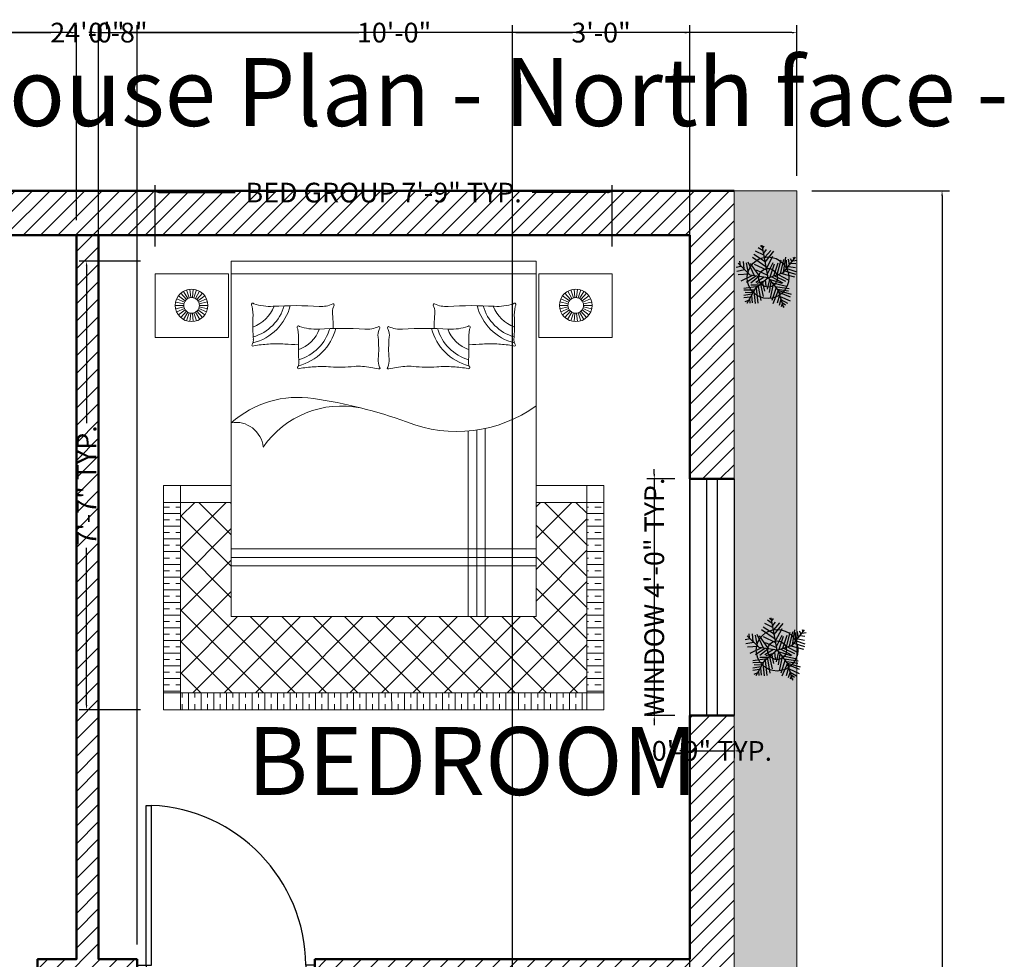
# Model space of a CAD drawing. Units: inches. Extents: x 1265938 to 1266301, y 2357745 to 2358240.
# Tile 4 of 4: x 1266101 to 1266301, y 2358050 to 2358240. Entities that reach past the tile are written whole.
import ezdxf

# ---------------------------------------------------------------- set-up
doc = ezdxf.new("R2010")
doc.units = ezdxf.units.IN
doc.header["$MEASUREMENT"] = 0
for name, color, linetype, lineweight in [('A-ANNO-TEXT', 7, 'Continuous', 25), ('A-AREA-IDEN', 7, 'Continuous', 18), ('A-DOOR', 4, 'Continuous', 25), ('A-FURN', 8, 'Continuous', 18), ('A-WALL-PATT', 8, 'Continuous', 13), ('L-PLNT', 3, 'Continuous', 18), ('L-PLNT-BEDS', 3, 'Continuous', 18), ('L-PLNT-PATT', 3, 'Continuous', 13), ('WALL', 7, 'Continuous', 50), ('WINDOW', 2, 'Continuous', 25), ('YQ_DIM', 3, 'Continuous', 18)]:
    doc.layers.add(name, color=color, linetype=linetype, lineweight=lineweight)
doc.layers.add('Layer2', color=102, linetype='Continuous')
doc.layers.add('RAMP SLOPE', color=8, linetype='Continuous')
doc.styles.get("Standard").update_dxf_attribs({"font": 'arial.ttf'})
doc.styles.add('YQ_DIM', font='SUPEROS.SHX', dxfattribs={"width": 0.8, "bigfont": 'HZDX.SHX'})
doc.dimstyles.new('yqi0', dxfattribs={"dimscale": 0, "dimtxt": 4, "dimasz": 1, "dimexe": 1.5, "dimexo": 3, "dimgap": 0.5, "dimtad": 0, "dimdsep": 46, "dimlunit": 4, "dimtxsty": 'Standard', "dimcen": 0, "dimclrd": 256, "dimclre": 256, "dimclrt": 7, "dimadec": 1, "dimazin": 2, "dimtfac": 1, "dimtix": 1, "dimtmove": 2, "dimatfit": 2, "dimfxl": 1, "dimtolj": 1, "dimtzin": 0, "dimarcsym": 0})

# ---------------------------------------------------------------- blocks, each defined once
blk = doc.blocks.new('WD_WIN4')
for p, q in [((-0.5, 0.5), (0.5, 0.5)), ((-0.5, 0.12), (0.5, 0.12)), ((-0.5, -0.12), (0.5, -0.12)), ((-0.5, -0.5), (0.5, -0.5))]:
    blk.add_line(p, q)
blk = doc.blocks.new('DR_D01')
for p, q in [((-0.45, 0.93), (-0.42, 0.93)), ((-0.45, 0.03), (-0.45, 0.93)), ((-0.42, 0.03), (-0.42, 0.93)), ((-0.5, 0.03), (-0.42, 0.03)), ((-0.5, 0.03), (-0.5, -0.03)), ((-0.45, 0.03), (-0.45, 0)), ((-0.45, 0), (-0.435, 0)), ((-0.435, 0), (-0.435, -0.03)), ((0.435, 0), (0.435, -0.03)), ((0.45, 0), (0.435, 0)), ((0.45, 0.03), (0.45, 0)), ((0.5, 0.03), (0.45, 0.03)), ((0.5, -0.03), (0.5, 0.03)), ((-0.435, -0.03), (-0.5, -0.03)), ((0.435, -0.03), (0.5, -0.03))]:
    blk.add_line(p, q)
blk.add_arc((-0.4602, 0.0206), 0.9103, 0.5915, 87.4664)
blk = doc.blocks.new('Trees - Metric')
at = {"layer": 'Layer2'}
for p, q in [((-221.9198, 1197.3052), (-433.5526, 1338.8594)), ((-258.7244, 1362.456), (-332.3336, 1421.4348)), ((0, 0), (-266.7, 1447.8)), ((-231.1146, 1315.2628), (-166.7002, 1421.4348)), ((-93.091, 489.5342), (-700.3796, 902.3858)), ((-129.8956, 713.6638), (-626.7704, 1032.1544)), ((-185.1152, 1008.5578), (-553.1612, 1185.4942)), ((-194.31, 1102.9442), (-65.4812, 1256.284)), ((-148.3106, 914.1968), (118.5418, 1220.9018)), ((-129.8956, 701.8528), (265.7602, 1185.4942)), ((-74.7014, 418.7444), (219.7608, 961.39)), ((685.8, 228.6), (1219.2, 914.4)), ((689.0258, 230.0224), (790.2448, 914.1968)), ((1121.4862, 925.9824), (1149.0706, 831.6214)), ((-1206.4492, 501.3198), (-1418.082, 465.9376)), ((-800.1, 114.3), (-1333.5, 647.7)), ((-1234.059, 536.7274), (-1252.4486, 737.2604)), ((-1105.2302, 725.4494), (-1077.6458, 395.1732)), ((-976.4268, 666.4706), (-884.4026, 194.6402)), ((-902.8176, 713.6638), (-617.5756, 100.2538)), ((-369.1382, 53.086), (-783.1836, 642.874)), ((-617.5756, 607.4918), (-74.7014, 347.98)), ((-28.6766, 171.0436), (228.9556, 678.2816)), ((100.1268, 41.275), (284.1498, 619.2774)), ((256.5654, 88.4682), (449.7832, 666.4706)), ((412.9786, 147.447), (587.8068, 796.2392)), ((560.197, 182.8292), (698.2206, 819.8358)), ((808.6344, 784.4282), (827.0494, 418.7444)), ((891.4384, 831.6214), (946.658, 572.1096)), ((919.0482, 501.3198), (1222.6798, 454.152)), ((983.4626, 867.0036), (1066.2666, 725.4494)), ((1029.462, 654.685), (1241.0948, 631.0884)), ((1112.2914, 760.8316), (1296.3144, 784.4282)), ((-1031.621, 347.98), (-1399.667, 277.1902)), ((-847.598, 159.2326), (-1326.0578, 135.636)), ((-718.7946, 88.4682), (-1215.644, -147.447)), ((-543.9664, 76.6572), (-967.2066, -206.4512)), ((0, 0), (-800.1, 114.3)), ((-405.9428, 53.086), (-764.794, -241.8334)), ((0, 0), (-571.5, -495.3)), ((-166.7002, 29.4894), (-543.9664, -206.4512)), ((-525.5514, 347.98), (-28.6766, 123.8504)), ((0, 0), (685.8, 228.6)), ((0, 0), (457.2, -571.5)), ((164.5412, 41.275), (661.416, -218.2368)), ((284.1498, 88.4682), (781.0246, -147.447)), ((458.978, 147.447), (891.4384, -88.4682)), ((615.4166, 194.6402), (1185.8752, 41.275)), ((753.4148, 312.5978), (1222.6798, 159.2326)), ((845.439, 418.7444), (1241.0948, 277.1902)), ((-442.7474, -383.3876), (-1086.8406, -477.7486)), ((-387.5278, -324.4088), (-764.794, -324.4088)), ((-166.7002, -147.447), (-507.1618, -253.619)), ((-433.5526, -383.3876), (-323.1134, -1020.3688)), ((-341.5284, -289.0012), (-221.9198, -831.6214)), ((-240.3094, -218.2368), (-157.5054, -595.7062)), ((-120.7008, -88.4682), (-93.091, -371.5766)), ((63.3222, -76.6826), (-37.8714, -513.1308)), ((44.9326, -64.897), (615.4166, -241.8334)), ((127.7366, -159.258), (54.1274, -654.685)), ((228.9556, -289.0012), (90.932, -914.1968)), ((357.759, -430.5554), (164.5412, -1020.3688)), ((192.151, -230.0224), (817.8292, -371.5766)), ((311.7596, -383.3876), (937.4378, -477.7486)), ((-718.7946, -737.2604), (-1086.8406, -796.2392)), ((-617.5756, -548.5384), (-1077.6458, -560.324)), ((-783.1836, -867.029), (-1077.6458, -902.4112)), ((-681.9646, -666.496), (-1022.4262, -654.685)), ((-571.5, -495.3), (-952.5, -1143)), ((-737.1842, -784.4536), (-709.5744, -1114.7298)), ((-635.9652, -607.5172), (-580.771, -1150.1374)), ((-525.5514, -465.963), (-451.9422, -1126.5408)), ((458.978, -572.1096), (210.5406, -1161.923)), ((514.1976, -772.6426), (403.7838, -1138.3264)), ((412.9786, -501.3452), (919.0482, -583.9206)), ((457.2, -571.5), (685.8, -1333.5)), ((468.1982, -572.1096), (1029.462, -737.2604)), ((486.5878, -642.8994), (983.4626, -843.4324)), ((541.8074, -831.6214), (992.6574, -1032.1544)), ((-875.2078, -1008.5832), (-1040.8412, -1079.3476)), ((-829.2084, -937.7934), (-810.7934, -1126.5408)), ((578.612, -961.39), (495.7826, -1232.7128)), ((578.612, -973.1756), (873.0488, -1138.3264)), ((624.6114, -1161.923), (587.8068, -1291.6916)), ((624.6114, -1102.9442), (781.0246, -1209.1162)), ((679.8056, -1268.095), (716.6102, -1291.6916))]:
    blk.add_line(p, q, dxfattribs=at)
blk = doc.blocks.new('A$Cbdbf8f2b')
at = {"layer": 'RAMP SLOPE'}
for radius in [7.17, 3.22]:
    blk.add_circle((13.77, 14.11), radius, dxfattribs=at)
at = {"xscale": 0.0077264756515533, "yscale": 0.0077264756515533, "zscale": 0.0077264756515533}
blk.add_blockref('Trees - Metric', (13.77, 14.11), dxfattribs=at)
blk = doc.blocks.new('BED')
h = blk.add_hatch()
h.set_pattern_fill('TRANS', color=256, scale=12, style=0)
h.set_pattern_definition([(360, (4433.967, -9715.0492), (1e-15, 3), []), (360, (4433.967, -9713.5492), (1e-15, 3), [1.5, -1.5])])
h.paths.add_polyline_path([(48, -103), (52, -103), (52, -58), (48, -58)])
h.paths.add_polyline_path([(-48, -58), (-52, -58), (-52, -103), (-48, -103)])
h = blk.add_hatch()
h.set_pattern_fill('ANSI37', color=256, scale=42, angle=-90, style=0)
h.set_pattern_definition([(315, (7787.1367, 4477.8466), (3.7123106, 3.7123106), []), (45, (7787.1367, 4477.8466), (-3.7123106, 3.7123106), [])])
h.paths.add_polyline_path([(-36, -85), (-36, -58), (-48, -58), (-48, -103), (48, -103), (48, -58), (36, -58), (36, -85)])
h = blk.add_hatch()
h.set_pattern_fill('TRANS', color=256, scale=12, angle=-90, style=0)
h.set_pattern_definition([(270, (4433.967, -9715.0492), (3, -1e-15), []), (270, (4435.467, -9715.0492), (3, -1e-15), [1.5, -1.5])])
h.paths.add_polyline_path([(48, -107), (48, -103), (-48, -103), (-48, -107)])
for p, q in [((-36, -1), (36, -1)), ((-36, -85), (-36, -1)), ((36, -1), (36, -85)), ((-54, -4), (-54, -19)), ((-36.64, -4), (-54, -4)), ((-36.64, -4), (-36.64, -19)), ((-36, -4), (36, -4)), ((36.64, -4), (36.64, -19)), ((36.64, -4), (54, -4)), ((54, -4), (54, -19)), ((-46.88, -10.37), (-48.5, -9.2)), ((-46.62, -10.08), (-47.96, -8.6)), ((-46.31, -9.86), (-47.31, -8.13)), ((-45.96, -9.7), (-46.58, -7.8)), ((-45.58, -9.62), (-45.8, -7.63)), ((-45.2, -9.62), (-45, -7.63)), ((-44.82, -9.7), (-44.21, -7.79)), ((-44.47, -9.85), (-43.48, -8.12)), ((-44.16, -10.08), (-42.83, -8.59)), ((-43.9, -10.36), (-42.29, -9.18)), ((43.9, -10.36), (42.29, -9.18)), ((44.16, -10.08), (42.83, -8.59)), ((44.47, -9.85), (43.48, -8.12)), ((44.82, -9.7), (44.21, -7.79)), ((45.2, -9.62), (45, -7.63)), ((45.58, -9.62), (45.8, -7.63)), ((45.96, -9.7), (46.58, -7.8)), ((46.31, -9.86), (47.31, -8.13)), ((46.62, -10.08), (47.96, -8.6)), ((46.88, -10.37), (48.5, -9.2)), ((-47.23, -11.45), (-49.23, -11.45)), ((-47.19, -11.07), (-49.14, -10.66)), ((-47.07, -10.7), (-48.9, -9.89)), ((-43.71, -10.7), (-41.89, -9.88)), ((-43.59, -11.06), (-41.64, -10.64)), ((-43.55, -11.44), (-41.55, -11.44)), ((43.55, -11.44), (41.55, -11.44)), ((43.59, -11.06), (41.64, -10.64)), ((43.71, -10.7), (41.89, -9.88)), ((47.07, -10.7), (48.9, -9.89)), ((47.19, -11.07), (49.14, -10.66)), ((47.23, -11.45), (49.23, -11.45)), ((-47.19, -11.83), (-49.14, -12.25)), ((-47.07, -12.2), (-48.89, -13.01)), ((-46.87, -12.53), (-48.49, -13.71)), ((-46.62, -12.81), (-47.95, -14.3)), ((-46.3, -13.04), (-47.3, -14.77)), ((-45.95, -13.2), (-46.57, -15.1)), ((-45.58, -13.27), (-45.78, -15.26)), ((-45.19, -13.27), (-44.98, -15.26)), ((-44.82, -13.19), (-44.2, -15.09)), ((-44.47, -13.04), (-43.46, -14.77)), ((-44.16, -12.81), (-42.82, -14.29)), ((-43.9, -12.52), (-42.28, -13.7)), ((-43.71, -12.19), (-41.88, -13)), ((-43.59, -11.83), (-41.63, -12.24)), ((43.59, -11.83), (41.63, -12.24)), ((43.71, -12.19), (41.88, -13)), ((43.9, -12.52), (42.28, -13.7)), ((44.16, -12.81), (42.82, -14.29)), ((44.47, -13.04), (43.46, -14.77)), ((44.82, -13.19), (44.2, -15.09)), ((45.19, -13.27), (44.98, -15.26)), ((45.58, -13.27), (45.78, -15.26)), ((45.95, -13.2), (46.57, -15.1)), ((46.3, -13.04), (47.3, -14.77)), ((46.62, -12.81), (47.95, -14.3)), ((46.87, -12.53), (48.49, -13.71)), ((47.07, -12.2), (48.89, -13.01)), ((47.19, -11.83), (49.14, -12.25)), ((-36.64, -19), (-54, -19)), ((36.64, -19), (54, -19)), ((20, -85), (20, -41.14)), ((22, -85), (22, -40.91)), ((24, -85), (24, -40.55)), ((-52, -54), (-52, -107)), ((-52, -54), (-36, -54)), ((-48, -54), (-48, -107)), ((36, -54), (52, -54)), ((48, -54), (48, -107)), ((52, -54), (52, -107)), ((-52, -58), (-36, -58)), ((36, -58), (52, -58)), ((36, -69), (-36, -69)), ((36, -71), (-36, -71)), ((36, -73), (-36, -73)), ((36, -85), (-36, -85)), ((-52, -103), (52, -103)), ((-52, -107), (52, -107))]:
    blk.add_line(p, q)
for centre, radius in [((-45.39, -11.45), 3.84), ((45.39, -11.45), 3.84), ((-45.39, -11.45), 1.84), ((45.39, -11.45), 1.84)]:
    blk.add_circle(centre, radius)
for centre, radius, start, end in [((-30.92, -11.24), 0.328, 35.8976, 208.6272), ((-42.38, -17.5), 12.73, 27.1629, 28.6272), ((-33.8, -8.61), 12.06, 283.8498, 346.0842), ((-33.8, -8.61), 10.71, 286.0319, 344.1205), ((-26.84, 0.13), 11.82, 251.1782, 273.3982), ((-20.92, -99.64), 88.13, 86.2964, 93.3982), ((-14.79, -4.98), 6.73, 266.2964, 294.303), ((-11.92, -11.33), 0.242, 335.7259, 114.303), ((-5.69, -14.14), 6.59, 155.7259, 159.0146), ((11.92, -11.33), 0.242, 65.697, 204.2741), ((5.69, -14.14), 6.59, 20.9854, 24.2741), ((14.79, -4.98), 6.73, 245.697, 273.7036), ((20.92, -99.64), 88.13, 86.6018, 93.7036), ((33.8, -8.61), 12.06, 193.9158, 256.1502), ((33.8, -8.61), 10.71, 195.8795, 253.9681), ((26.84, 0.13), 11.82, 266.6018, 288.8218), ((30.92, -11.24), 0.328, 331.3728, 144.1024), ((42.38, -17.5), 12.73, 151.3728, 152.8371), ((-44.37, -13.89), 13.5, 357.4804, 9.3956), ((-33.8, -8.61), 8.46, 289.8695, 338.9843), ((-8.24, -13.16), 3.86, 159.0146, 186.273), ((-36.64, -16.28), 24.71, 358.5721, 6.273), ((8.24, -13.16), 3.86, 353.727, 20.9854), ((36.64, -16.28), 24.71, 173.727, 181.4279), ((33.8, -8.61), 8.46, 201.0157, 250.1305), ((44.37, -13.89), 13.5, 170.6044, 182.5196), ((10.15, -16.29), 41.07, 177.4804, 184.5075), ((-10.15, -16.29), 41.07, 355.4925, 2.5196), ((-20.16, -16.62), 0.328, 35.8976, 208.6272), ((-31.62, -22.87), 12.73, 27.1629, 28.6272), ((-33.61, -19.26), 13.5, 357.4804, 9.3956), ((-23.04, -13.99), 8.46, 289.8695, 338.9843), ((-23.04, -13.99), 12.06, 283.8498, 346.0842), ((-23.04, -13.99), 10.71, 286.0319, 344.1205), ((-16.08, -5.24), 11.82, 251.1782, 273.3982), ((-10.15, -105.01), 88.13, 86.2964, 93.3982), ((-4.03, -10.35), 6.73, 266.2964, 294.303), ((2.52, -18.53), 3.86, 159.0146, 186.273), ((-1.16, -16.7), 0.242, 335.7259, 114.303), ((5.07, -19.51), 6.59, 155.7259, 159.0146), ((1.16, -16.7), 0.242, 65.697, 204.2741), ((-5.07, -19.51), 6.59, 20.9854, 24.2741), ((-2.52, -18.53), 3.86, 353.727, 20.9854), ((4.03, -10.35), 6.73, 245.697, 273.7036), ((10.15, -105.01), 88.13, 86.6018, 93.7036), ((23.04, -13.99), 12.06, 193.9158, 256.1502), ((23.04, -13.99), 10.71, 195.8795, 253.9681), ((23.04, -13.99), 8.46, 201.0157, 250.1305), ((16.08, -5.24), 11.82, 266.6018, 288.8218), ((20.16, -16.62), 0.328, 331.3728, 144.1024), ((33.61, -19.26), 13.5, 170.6044, 182.5196), ((31.62, -22.87), 12.73, 151.3728, 152.8371), ((-30.88, -20.82), 0.25, 147.6219, 311.9343), ((-32.72, -19.65), 1.93, 327.6219, 339.2246), ((-32.67, -19.67), 1.88, 339.2246, 4.5075), ((-25.16, -53.53), 33, 93.5164, 99.6766), ((-25.27, -51.86), 31.33, 86.4836, 93.5164), ((-21.12, 15.68), 36.34, 266.4836, 271.5234), ((20.91, -21.66), 41.07, 177.4804, 184.5075), ((-25.88, -21.66), 24.71, 354.3784, 6.273), ((25.88, -21.66), 24.71, 173.727, 185.6216), ((-20.91, -21.66), 41.07, 355.4925, 2.5196), ((21.12, 15.68), 36.34, 268.4766, 273.5164), ((25.27, -51.86), 31.33, 86.4836, 93.5164), ((25.16, -53.53), 33, 80.3234, 86.4836), ((30.88, -20.82), 0.25, 228.0657, 32.3781), ((32.67, -19.67), 1.88, 175.4925, 200.7754), ((32.72, -19.65), 1.93, 200.7754, 212.3781), ((-21.91, -25.04), 1.88, 339.2246, 4.5075), ((2.55, -24.46), 3.86, 174.3784, 204.7617), ((-2.55, -24.46), 3.86, 335.2383, 5.6216), ((21.91, -25.04), 1.88, 175.4925, 200.7754), ((-20.12, -26.19), 0.25, 147.6219, 311.9343), ((-21.96, -25.02), 1.93, 327.6219, 339.2246), ((-14.4, -58.9), 33, 93.5164, 99.6766), ((-14.51, -57.23), 31.33, 86.4836, 93.5164), ((-10.35, 10.3), 36.34, 266.4836, 275.306), ((-5.78, -38.98), 13.15, 77.9645, 95.306), ((2.5, -0.17), 26.53, 257.9645, 261.9243), ((-1.09, -26.25), 0.228, 231.9005, 52.8902), ((1.09, -26.25), 0.228, 127.1098, 308.0995), ((-2.5, -0.17), 26.53, 278.0757, 282.0355), ((5.78, -38.98), 13.15, 84.694, 102.0355), ((10.35, 10.3), 36.34, 264.694, 273.5164), ((14.51, -57.23), 31.33, 86.4836, 93.5164), ((14.4, -58.9), 33, 80.3234, 86.4836), ((20.12, -26.19), 0.25, 228.0657, 32.3781), ((21.96, -25.02), 1.93, 200.7754, 212.3781), ((-20.27, -56.85), 23.66, 81.0857, 131.6581), ((-32.56, -143.87), 111.55, 70.0977, 81.7735), ((-9.91, -57.83), 22.61, 78.6456, 145.1521), ((17.27, -9.21), 32.05, 248.2778, 305.7663), ((-34.97, -45.63), 6.55, 6.3172, 99.0807)]:
    blk.add_arc(centre, radius, start, end)
blk = doc.blocks.new('*D18')
at = {"layer": 'Defpoints', "color": 0, "transparency": 16777216}
for p in [(1266221.65, 2358205.3), (1266128.88, 2358191.38), (1266221.65, 2358191.38)]:
    blk.add_point(p, dxfattribs=at)
at = {"layer": 'YQ_DIM', "lineweight": -2, "transparency": 16777216}
for p, q in [((1266128.88, 2358194.38), (1266128.88, 2358206.8)), ((1266221.65, 2358194.38), (1266221.65, 2358206.8)), ((1266129.88, 2358205.3), (1266145.12, 2358205.3)), ((1266220.65, 2358205.3), (1266205.41, 2358205.3))]:
    blk.add_line(p, q, dxfattribs=at)
at = {"layer": 'YQ_DIM', "transparency": 16777216}
for points in [[(1266129.88, 2358205.46), (1266129.88, 2358205.13), (1266128.88, 2358205.3)], [(1266220.65, 2358205.46), (1266220.65, 2358205.13), (1266221.65, 2358205.3)]]:
    blk.add_solid(points, dxfattribs=at)
at = {"layer": 'YQ_DIM', "color": 7, "transparency": 16777216, "insert": (1266175.26, 2358205.3), "char_height": 4, "attachment_point": 5}
blk.add_mtext('\\A1;BED GROUP 7\'-9" TYP.', dxfattribs=at)
blk = doc.blocks.new('*D19')
at = {"layer": 'Defpoints', "color": 0, "transparency": 16777216}
for p in [(1266114.96, 2358191.38), (1266128.88, 2358191.38), (1266128.88, 2358100.33)]:
    blk.add_point(p, dxfattribs=at)
at = {"layer": 'YQ_DIM', "lineweight": -2, "transparency": 16777216}
for p, q in [((1266125.88, 2358191.38), (1266113.46, 2358191.38)), ((1266114.96, 2358190.38), (1266114.96, 2358158.53)), ((1266114.96, 2358101.33), (1266114.96, 2358133.18)), ((1266125.88, 2358100.33), (1266113.46, 2358100.33))]:
    blk.add_line(p, q, dxfattribs=at)
at = {"layer": 'YQ_DIM', "transparency": 16777216}
for points in [[(1266114.8, 2358190.38), (1266115.13, 2358190.38), (1266114.96, 2358191.38)], [(1266114.8, 2358101.33), (1266115.13, 2358101.33), (1266114.96, 2358100.33)]]:
    blk.add_solid(points, dxfattribs=at)
at = {"layer": 'YQ_DIM', "color": 7, "transparency": 16777216, "insert": (1266114.96, 2358145.86), "char_height": 4, "attachment_point": 5, "rotation": 90}
blk.add_mtext('\\A1;7\'-7" TYP.', dxfattribs=at)
blk = doc.blocks.new('*D20')
at = {"layer": 'Defpoints', "color": 0, "transparency": 16777216}
for p in [(1266237.39, 2358147.18), (1266230.19, 2358099.18), (1266237.39, 2358099.18)]:
    blk.add_point(p, dxfattribs=at)
at = {"layer": 'YQ_DIM', "lineweight": -2, "transparency": 16777216}
for p, q in [((1266230.19, 2358148.18), (1266230.19, 2358149.18)), ((1266234.39, 2358147.18), (1266228.69, 2358147.18)), ((1266230.19, 2358147.18), (1266230.19, 2358099.18)), ((1266234.39, 2358099.18), (1266228.69, 2358099.18)), ((1266230.19, 2358098.18), (1266230.19, 2358097.18))]:
    blk.add_line(p, q, dxfattribs=at)
at = {"layer": 'YQ_DIM', "transparency": 16777216}
for points in [[(1266230.02, 2358148.18), (1266230.36, 2358148.18), (1266230.19, 2358147.18)], [(1266230.02, 2358098.18), (1266230.36, 2358098.18), (1266230.19, 2358099.18)]]:
    blk.add_solid(points, dxfattribs=at)
at = {"layer": 'YQ_DIM', "color": 7, "transparency": 16777216, "insert": (1266230.19, 2358123.18), "char_height": 4, "attachment_point": 5, "rotation": 90}
blk.add_mtext('\\A1;WINDOW 4\'-0" TYP.', dxfattribs=at)
blk = doc.blocks.new('*D21')
at = {"layer": 'Defpoints', "color": 0, "transparency": 16777216}
for p in [(1266237.39, 2358099.18), (1266246.39, 2358099.18), (1266246.39, 2358091.98)]:
    blk.add_point(p, dxfattribs=at)
at = {"layer": 'YQ_DIM', "lineweight": -2, "transparency": 16777216}
for p, q in [((1266237.39, 2358096.18), (1266237.39, 2358090.48)), ((1266246.39, 2358096.18), (1266246.39, 2358090.48)), ((1266236.39, 2358091.98), (1266235.39, 2358091.98)), ((1266237.39, 2358091.98), (1266246.39, 2358091.98)), ((1266247.39, 2358091.98), (1266248.39, 2358091.98))]:
    blk.add_line(p, q, dxfattribs=at)
at = {"layer": 'YQ_DIM', "transparency": 16777216}
for points in [[(1266236.39, 2358092.15), (1266236.39, 2358091.81), (1266237.39, 2358091.98)], [(1266247.39, 2358092.15), (1266247.39, 2358091.81), (1266246.39, 2358091.98)]]:
    blk.add_solid(points, dxfattribs=at)
at = {"layer": 'YQ_DIM', "color": 7, "transparency": 16777216, "insert": (1266241.89, 2358091.98), "char_height": 4, "attachment_point": 5}
blk.add_mtext('\\A1;0\'-9" TYP.', dxfattribs=at)
blk = doc.blocks.new('*D34')
at = {"layer": 'Defpoints', "color": 0, "transparency": 16777216}
for p in [(1266259.14, 2358237.77), (1265971.14, 2358205.68), (1266259.14, 2358205.68)]:
    blk.add_point(p, dxfattribs=at)
at = {"layer": 'YQ_DIM', "lineweight": -2, "transparency": 16777216}
for p, q in [((1265971.14, 2358208.68), (1265971.14, 2358239.27)), ((1265972.14, 2358237.77), (1266107.74, 2358237.77)), ((1266258.14, 2358237.77), (1266122.54, 2358237.77)), ((1266259.14, 2358208.68), (1266259.14, 2358239.27))]:
    blk.add_line(p, q, dxfattribs=at)
at = {"layer": 'YQ_DIM', "transparency": 16777216}
for points in [[(1265972.14, 2358237.93), (1265972.14, 2358237.6), (1265971.14, 2358237.77)], [(1266258.14, 2358237.93), (1266258.14, 2358237.6), (1266259.14, 2358237.77)]]:
    blk.add_solid(points, dxfattribs=at)
at = {"layer": 'YQ_DIM', "color": 7, "transparency": 16777216, "insert": (1266115.14, 2358237.77), "char_height": 4, "attachment_point": 5}
blk.add_mtext('\\A1;24\'-0"', dxfattribs=at)
blk = doc.blocks.new('*D35')
at = {"layer": 'Defpoints', "color": 0, "transparency": 16777216}
for p in [(1266259.14, 2358205.68), (1266288.6, 2358205.68), (1266259.14, 2357797.68)]:
    blk.add_point(p, dxfattribs=at)
at = {"layer": 'YQ_DIM', "lineweight": -2, "transparency": 16777216}
for p, q in [((1266262.14, 2358205.68), (1266290.1, 2358205.68)), ((1266288.6, 2358204.68), (1266288.6, 2358009.05)), ((1266288.6, 2357798.68), (1266288.6, 2357994.31)), ((1266262.14, 2357797.68), (1266290.1, 2357797.68))]:
    blk.add_line(p, q, dxfattribs=at)
at = {"layer": 'YQ_DIM', "transparency": 16777216}
for points in [[(1266288.44, 2358204.68), (1266288.77, 2358204.68), (1266288.6, 2358205.68)], [(1266288.44, 2357798.68), (1266288.77, 2357798.68), (1266288.6, 2357797.68)]]:
    blk.add_solid(points, dxfattribs=at)
at = {"layer": 'YQ_DIM', "color": 7, "transparency": 16777216, "insert": (1266288.6, 2358001.68), "char_height": 4, "attachment_point": 5, "rotation": 90}
blk.add_mtext('\\A1;34\'-0"', dxfattribs=at)
blk = doc.blocks.new('*D38')
at = {"layer": 'Defpoints', "color": 0, "transparency": 16777216}
for p in [(1266112.89, 2358237.77), (1265992.89, 2358196.68), (1266112.89, 2358196.68)]:
    blk.add_point(p, dxfattribs=at)
at = {"layer": 'YQ_DIM', "lineweight": -2, "transparency": 16777216}
for p, q in [((1265992.89, 2358199.68), (1265992.89, 2358239.27)), ((1265993.89, 2358237.77), (1266045.71, 2358237.77)), ((1266111.89, 2358237.77), (1266060.07, 2358237.77)), ((1266112.89, 2358199.68), (1266112.89, 2358239.27))]:
    blk.add_line(p, q, dxfattribs=at)
at = {"layer": 'YQ_DIM', "transparency": 16777216}
for points in [[(1265993.89, 2358237.93), (1265993.89, 2358237.6), (1265992.89, 2358237.77)], [(1266111.89, 2358237.93), (1266111.89, 2358237.6), (1266112.89, 2358237.77)]]:
    blk.add_solid(points, dxfattribs=at)
at = {"layer": 'YQ_DIM', "color": 7, "transparency": 16777216, "insert": (1266052.89, 2358237.77), "char_height": 4, "attachment_point": 5}
blk.add_mtext('\\A1;10\'-0"', dxfattribs=at)
blk = doc.blocks.new('*D39')
at = {"layer": 'Defpoints', "color": 0, "transparency": 16777216}
for p in [(1266237.39, 2358237.77), (1266117.39, 2358196.68), (1266237.39, 2358196.68)]:
    blk.add_point(p, dxfattribs=at)
at = {"layer": 'YQ_DIM', "lineweight": -2, "transparency": 16777216}
for p, q in [((1266117.39, 2358199.68), (1266117.39, 2358239.27)), ((1266118.39, 2358237.77), (1266170.21, 2358237.77)), ((1266236.39, 2358237.77), (1266184.57, 2358237.77)), ((1266237.39, 2358199.68), (1266237.39, 2358239.27))]:
    blk.add_line(p, q, dxfattribs=at)
at = {"layer": 'YQ_DIM', "transparency": 16777216}
for points in [[(1266118.39, 2358237.93), (1266118.39, 2358237.6), (1266117.39, 2358237.77)], [(1266236.39, 2358237.93), (1266236.39, 2358237.6), (1266237.39, 2358237.77)]]:
    blk.add_solid(points, dxfattribs=at)
at = {"layer": 'YQ_DIM', "color": 7, "transparency": 16777216, "insert": (1266177.39, 2358237.77), "char_height": 4, "attachment_point": 5}
blk.add_mtext('\\A1;10\'-0"', dxfattribs=at)
blk = doc.blocks.new('*D47')
at = {"layer": 'Defpoints', "color": 0, "transparency": 16777216}
for p in [(1266201.39, 2358237.77), (1266201.39, 2357818.68), (1266237.39, 2357818.68)]:
    blk.add_point(p, dxfattribs=at)
at = {"layer": 'YQ_DIM', "lineweight": -2, "transparency": 16777216}
for p, q in [((1266201.39, 2357821.68), (1266201.39, 2358239.27)), ((1266202.39, 2358237.77), (1266213.58, 2358237.77)), ((1266236.39, 2358237.77), (1266225.21, 2358237.77)), ((1266237.39, 2357821.68), (1266237.39, 2358239.27))]:
    blk.add_line(p, q, dxfattribs=at)
at = {"layer": 'YQ_DIM', "transparency": 16777216}
for points in [[(1266202.39, 2358237.93), (1266202.39, 2358237.6), (1266201.39, 2358237.77)], [(1266236.39, 2358237.93), (1266236.39, 2358237.6), (1266237.39, 2358237.77)]]:
    blk.add_solid(points, dxfattribs=at)
at = {"layer": 'YQ_DIM', "color": 7, "transparency": 16777216, "insert": (1266219.39, 2358237.77), "char_height": 4, "attachment_point": 5}
blk.add_mtext('\\A1;3\'-0"', dxfattribs=at)
blk = doc.blocks.new('*D49')
at = {"layer": 'Defpoints', "color": 0, "transparency": 16777216}
for p in [(1266125.26, 2358237.77), (1266117.39, 2358049.68), (1266125.26, 2358049.68)]:
    blk.add_point(p, dxfattribs=at)
at = {"layer": 'YQ_DIM', "lineweight": -2, "transparency": 16777216}
for p, q in [((1266116.39, 2358237.77), (1266115.39, 2358237.77)), ((1266117.39, 2358052.68), (1266117.39, 2358239.27)), ((1266117.39, 2358237.77), (1266125.26, 2358237.77)), ((1266125.26, 2358052.68), (1266125.26, 2358239.27)), ((1266126.26, 2358237.77), (1266127.26, 2358237.77))]:
    blk.add_line(p, q, dxfattribs=at)
at = {"layer": 'YQ_DIM', "transparency": 16777216}
for points in [[(1266116.39, 2358237.93), (1266116.39, 2358237.6), (1266117.39, 2358237.77)], [(1266126.26, 2358237.93), (1266126.26, 2358237.6), (1266125.26, 2358237.77)]]:
    blk.add_solid(points, dxfattribs=at)
at = {"layer": 'YQ_DIM', "color": 7, "transparency": 16777216, "insert": (1266121.33, 2358237.77), "char_height": 4, "attachment_point": 5}
blk.add_mtext('\\A1;0\'-8"', dxfattribs=at)

msp = doc.modelspace()

# ---------------------------------------------------------------- hatches: boundary and pattern name
at = {"layer": 'A-WALL-PATT'}
h = msp.add_hatch(dxfattribs=at)
h.set_pattern_fill('ANSI31', color=256, scale=20)
h.paths.add_polyline_path([(1266246.39, 2358205.681), (1265983.89, 2358205.681), (1265983.89, 2358147.181), (1265992.89, 2358147.181), (1265992.89, 2358196.681), (1266112.89, 2358196.681), (1266119.229, 2358196.681), (1266237.39, 2358196.681), (1266237.39, 2358147.181), (1266246.39, 2358147.181)])
h = msp.add_hatch(dxfattribs=at)
h.set_pattern_fill('ANSI31', color=256, scale=20)
h.paths.add_polyline_path([(1266117.39, 2358196.681), (1266112.89, 2358196.681), (1266112.89, 2358049.681), (1266105.016, 2358049.681), (1266105.016, 2358045.181), (1266125.264, 2358045.181), (1266125.264, 2358049.681), (1266117.39, 2358049.681)])
h = msp.add_hatch(dxfattribs=at)
h.set_pattern_fill('ANSI31', color=256, scale=20)
h.paths.add_polyline_path([(1266069.016, 2358049.681), (1265992.89, 2358049.681), (1265992.89, 2358099.181), (1265983.89, 2358099.181), (1265983.89, 2358012.181), (1265992.89, 2358012.181), (1265992.89, 2358045.181), (1266069.016, 2358045.181)])
h.paths.add_polyline_path([(1266246.39, 2358049.681), (1266246.39, 2358099.181), (1266237.39, 2358099.181), (1266237.39, 2358049.681), (1266161.264, 2358049.681), (1266161.264, 2358045.181), (1266178.89, 2358045.181), (1266178.89, 2357987.055), (1266183.39, 2357987.055), (1266183.39, 2358045.181), (1266237.39, 2358045.181), (1266237.39, 2358029.655), (1266246.39, 2358029.655)])
h.paths.add_polyline_path([(1265992.89, 2357938.681), (1266058.89, 2357938.681), (1266058.89, 2357943.181), (1265992.89, 2357943.181), (1265992.89, 2357976.181), (1265983.89, 2357976.181), (1265983.89, 2357967.701), (1265984.307, 2357966.989), (1265983.89, 2357967.035), (1265983.89, 2357902.681), (1265992.89, 2357902.681)])
h.paths.add_polyline_path([(1266069.016, 2357943.181), (1266058.89, 2357943.181), (1266058.89, 2357938.681), (1266069.016, 2357938.681)])
h.paths.add_polyline_path([(1266125.264, 2357943.181), (1266105.016, 2357943.181), (1266105.016, 2357938.681), (1266112.89, 2357938.681), (1266112.89, 2357818.681), (1266105.024, 2357818.681), (1266105.024, 2357809.681), (1266112.898, 2357809.681), (1266153.39, 2357809.681), (1266153.39, 2357818.681), (1266117.39, 2357818.681), (1266117.39, 2357938.681), (1266125.264, 2357938.681)])
h.paths.add_polyline_path([(1266069.024, 2357818.681), (1265999.055, 2357818.681), (1265992.89, 2357818.681), (1265992.89, 2357854.681), (1265983.89, 2357854.681), (1265983.89, 2357809.681), (1266069.024, 2357809.681)])
h.paths.add_polyline_path([(1266246.39, 2358005.655), (1266237.39, 2358005.655), (1266237.39, 2357943.181), (1266161.264, 2357943.181), (1266161.264, 2357938.681), (1266237.39, 2357938.681), (1266237.39, 2357818.681), (1266201.39, 2357818.681), (1266201.39, 2357809.681), (1266246.39, 2357809.681)])
at = {"layer": 'L-PLNT-PATT'}
h = msp.add_hatch(dxfattribs=at)
h.set_pattern_fill('GRASS', color=256, scale=4)
h.paths.add_polyline_path([(1266259.14, 2358205.681), (1266246.39, 2358205.681), (1266246.39, 2358099.181), (1266246.39, 2358049.681), (1266246.39, 2357797.681), (1266259.14, 2357797.681), (1266259.14, 2358049.681)])

# ---------------------------------------------------------------- linework, layer by layer
at = {"layer": 'L-PLNT-BEDS'}
msp.add_lwpolyline([(1266246.39, 2357797.681), (1266246.39, 2358049.681), (1266246.39, 2358099.181), (1266246.39, 2358205.681), (1266259.14, 2358205.681), (1266259.14, 2358049.681), (1266259.14, 2357797.681)], close=True, dxfattribs=at)
at = {"layer": 'WALL'}
for p, q in [((1265992.89, 2358196.681), (1266112.89, 2358196.681)), ((1266117.39, 2358196.681), (1266237.39, 2358196.681)), ((1266117.39, 2358196.681), (1266119.229, 2358196.681)), ((1266237.39, 2358147.181), (1266237.39, 2358196.681)), ((1266237.39, 2358147.181), (1266246.39, 2358147.181)), ((1266237.39, 2358049.681), (1266237.39, 2358099.181)), ((1266237.39, 2358099.181), (1266246.39, 2358099.181)), ((1266161.264, 2358049.681), (1266237.39, 2358049.681)), ((1266161.264, 2358049.681), (1266161.264, 2358045.181))]:
    msp.add_line(p, q, dxfattribs=at)
msp.add_lwpolyline([(1265983.89, 2358205.681), (1266246.39, 2358205.681)], dxfattribs=at)
msp.add_lwpolyline([(1266125.264, 2358049.681), (1266117.39, 2358049.681), (1266117.39, 2358196.681), (1266112.89, 2358196.681), (1266112.89, 2358049.681), (1266105.016, 2358049.681), (1266105.016, 2358045.181), (1266125.264, 2358045.181)], close=True, dxfattribs=at)

# ---------------------------------------------------------------- block references
at = {"layer": 'A-DOOR', "xscale": 36, "yscale": 36, "zscale": 36}
msp.add_blockref('DR_D01', (1266143.264, 2358047.431), dxfattribs=at)
at = {"layer": 'A-FURN', "xscale": 0.858999246329296, "yscale": 0.858999246329296, "zscale": 0.858999246329296}
msp.add_blockref('BED', (1266175.264, 2358192.241), dxfattribs=at)
at = {"layer": 'L-PLNT', "xscale": 0.5886644209444821, "yscale": 0.5886644209444821, "zscale": 0.5886644209444821}
for p in [(1266245.173, 2358179.704), (1266247.011, 2358104.112)]:
    msp.add_blockref('A$Cbdbf8f2b', p, dxfattribs=at)
at = {"layer": 'WINDOW', "xscale": 48, "yscale": 9, "zscale": 48, "rotation": 270}
msp.add_blockref('WD_WIN4', (1266241.89, 2358123.181), dxfattribs=at)

# ---------------------------------------------------------------- texts
at = {"layer": 'A-ANNO-TEXT', "insert": (1265939.922, 2358232.591), "char_height": 13.77953, "width": 415.35736, "attachment_point": 1, "style": 'YQ_DIM'}
msp.add_mtext('24x34 (816 sq ft) House Plan - North face - FP1319', dxfattribs=at)
at = {"layer": 'A-AREA-IDEN', "insert": (1266160.935, 2358096.807), "char_height": 13.77953, "width": 64.71906, "attachment_point": 1, "style": 'YQ_DIM'}
msp.add_mtext('\\pxqc;BEDROOM', dxfattribs=at)

# ---------------------------------------------------------------- dimensions: what is measured, and where the dimension line sits
at = {"layer": 'YQ_DIM'}
for base, p1, p2, picture, middle in [((1266259.14, 2358237.768), (1265971.14, 2358205.681), (1266259.14, 2358205.681), '*D34', (1266115.14, 2358237.768)), ((1266112.89, 2358237.768), (1265992.89, 2358196.681), (1266112.89, 2358196.681), '*D38', (1266052.89, 2358237.768)), ((1266125.264, 2358237.768), (1266117.39, 2358049.681), (1266125.264, 2358049.681), '*D49', (1266121.327, 2358237.768)), ((1266237.39, 2358237.768), (1266117.39, 2358196.681), (1266237.39, 2358196.681), '*D39', (1266177.39, 2358237.768)), ((1266201.39, 2358237.768), (1266237.39, 2357818.681), (1266201.39, 2357818.681), '*D47', (1266219.39, 2358237.768))]:
    dim = msp.add_linear_dim(base=base, p1=p1, p2=p2, dimstyle='yqi0', override={"dimscale": 1, "dimdec": 1, "dimzin": 1, "dimfrac": 2}, dxfattribs=at)
    dim.commit()
    dim.dimension.update_dxf_attribs({"geometry": picture, "text_midpoint": middle})
for base, p1, p2, text, picture, middle in [((1266221.65, 2358205.298), (1266128.879, 2358191.382), (1266221.65, 2358191.382), 'BED GROUP <> TYP.', '*D18', (1266175.264, 2358205.298)), ((1266246.39, 2358091.981), (1266237.39, 2358099.181), (1266246.39, 2358099.181), '<> TYP.', '*D21', (1266241.89, 2358091.981))]:
    dim = msp.add_linear_dim(base=base, p1=p1, p2=p2, text=text, dimstyle='yqi0', override={"dimscale": 1, "dimdec": 1, "dimzin": 1, "dimfrac": 2}, dxfattribs=at)
    dim.commit()
    dim.dimension.update_dxf_attribs({"geometry": picture, "text_midpoint": middle})
dim = msp.add_linear_dim(base=(1266288.602, 2358205.681), p1=(1266259.14, 2357797.681), p2=(1266259.14, 2358205.681), angle=90, dimstyle='yqi0', override={"dimscale": 1, "dimdec": 1, "dimzin": 1, "dimfrac": 2}, dxfattribs=at)
dim.commit()
dim.dimension.update_dxf_attribs({"geometry": '*D35', "text_midpoint": (1266288.602, 2358001.681)})
for base, p1, p2, angle, text, picture, middle in [((1266114.963, 2358191.382), (1266128.879, 2358100.328), (1266128.879, 2358191.382), 90, '<> TYP.', '*D19', (1266114.963, 2358145.855)), ((1266230.19, 2358099.181), (1266237.39, 2358147.181), (1266237.39, 2358099.181), 270, 'WINDOW <> TYP.', '*D20', (1266230.19, 2358123.181))]:
    dim = msp.add_linear_dim(base=base, p1=p1, p2=p2, angle=angle, text=text, dimstyle='yqi0', override={"dimscale": 1, "dimdec": 1, "dimzin": 1, "dimfrac": 2}, dxfattribs=at)
    dim.commit()
    dim.dimension.update_dxf_attribs({"geometry": picture, "text_midpoint": middle})

doc.saveas('drawing.dxf')
